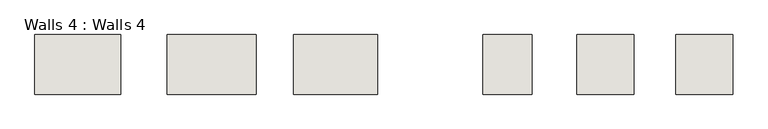
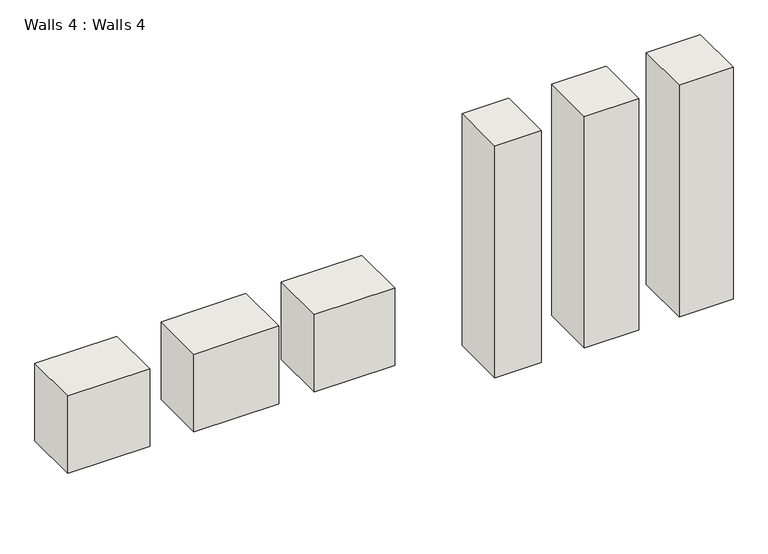
"""IFC4 building model written with IfcOpenShell, lengths in millimetres: wall geometry, Walls 4 : Walls 4."""

from ifc_helpers import new_model, si_unit, frame, origin, place, context, project, spatial, polyline, outline, extrude, source, transform, mapped, element, save


def walls_4_walls_4_5f3310eb(model_context):
    return source(origin(), model_context, "Body", "SweptSolid", [
        extrude(outline(polyline([(-7966.2326582, 3366.8419215), (-8271.0326582, 3366.8419215), (-8271.0326582, 3578.0277962), (-7966.2326582, 3578.0277962), (-7966.2326582, 3366.8419215)])), frame((0.0, 0.0, 11528.793472), z_axis=(0.0, 0.0, 1.0), x_axis=(1.0, 0.0, 0.0)), (0.0, 0.0, 1.0), 304.8),
        extrude(outline(polyline([(-7486.3936733, 3366.8419215), (-7802.0078801, 3366.8419215), (-7802.0078801, 3578.0277962), (-7486.3936733, 3578.0277962), (-7486.3936733, 3366.8419215)])), frame((0.0, 0.0, 11528.793472), z_axis=(0.0, 0.0, 1.0), x_axis=(1.0, 0.0, 0.0)), (0.0, 0.0, 1.0), 304.8),
        extrude(outline(polyline([(-7055.8320968, 3366.8419215), (-7354.3024101, 3366.8419215), (-7354.3024101, 3578.0277962), (-7055.8320968, 3578.0277962), (-7055.8320968, 3366.8419215)])), frame((0.0, 0.0, 11528.793472), z_axis=(0.0, 0.0, 1.0), x_axis=(1.0, 0.0, 0.0)), (0.0, 0.0, 1.0), 304.8),
        extrude(outline(polyline([(-6509.6914701, 3366.8419215), (-6682.7442051, 3366.8419215), (-6682.7442051, 3578.0277962), (-6509.6914701, 3578.0277962), (-6509.6914701, 3366.8419215)])), frame((0.0, 0.0, 11349.3315531), z_axis=(0.0, 0.0, 1.0), x_axis=(1.0, 0.0, 0.0)), (0.0, 0.0, 1.0), 910.9042063),
        extrude(outline(polyline([(-6147.2632325, 3366.8419215), (-6349.7966594, 3366.8419215), (-6349.7966594, 3578.0277962), (-6147.2632325, 3578.0277962), (-6147.2632325, 3366.8419215)])), frame((0.0, 0.0, 11349.3315531), z_axis=(0.0, 0.0, 1.0), x_axis=(1.0, 0.0, 0.0)), (0.0, 0.0, 1.0), 910.9042063),
        extrude(outline(polyline([(-5797.2936733, 3366.8419215), (-5998.0280758, 3366.8419215), (-5998.0280758, 3578.0277962), (-5797.2936733, 3578.0277962), (-5797.2936733, 3366.8419215)])), frame((0.0, 0.0, 11349.3315531), z_axis=(0.0, 0.0, 1.0), x_axis=(1.0, 0.0, 0.0)), (0.0, 0.0, 1.0), 910.9042063),
    ])


if __name__ == "__main__":
    model = new_model("IFC4")
    model_context = context("Model", 3, world=origin())
    ifc_project = project(units=[si_unit("LENGTHUNIT", "METRE", prefix="MILLI")], contexts=[model_context])
    site = spatial("IfcSite", under=ifc_project)
    building = spatial("IfcBuilding", under=site)
    placement = place(None, origin())
    walls_4_walls_4_shape = walls_4_walls_4_5f3310eb(model_context)
    element("IfcWall", 1, ObjectType="Walls 4 : Walls 4", at=placement, inside=building, context=model_context, shape_type="MappedRepresentation", body=[
        mapped(walls_4_walls_4_shape, transform((0.0, 0.0, 0.0), x_axis=(1.0, 0.0, 0.0), y_axis=(0.0, 1.0, 0.0), z_axis=(0.0, 0.0, 1.0))),
    ])
    save(model, "model.ifc")

# Revit data of these elements
# Element 1 (IfcWall, "Walls 4 : Walls 4")
#   Materials on its faces: "Default Wall"
# Materials
#   "Default Wall": colour RGB 128 128 128, transparency 0
